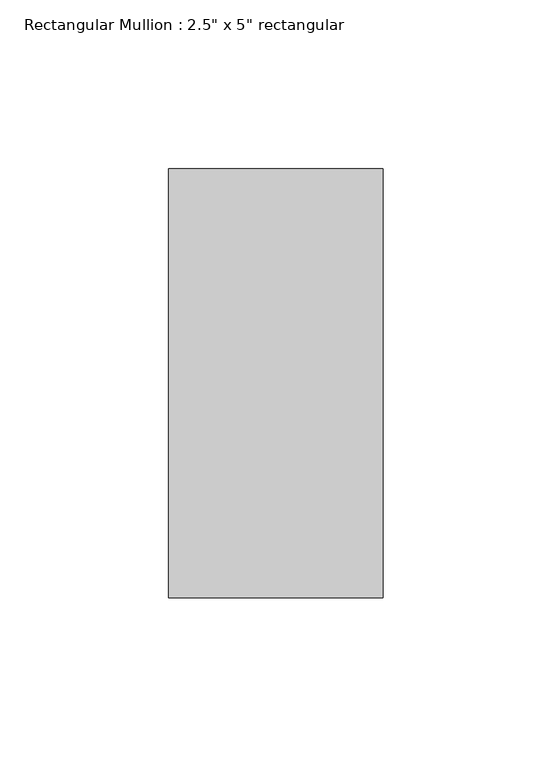
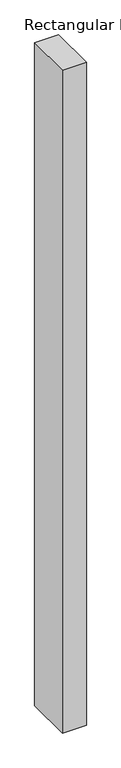
"""IFC4 building model written with IfcOpenShell, lengths in millimetres: member geometry."""

from ifc_helpers import new_model, si_unit, frame, origin, place, context, project, spatial, polyline, outline, extrude, source, transform, mapped, element, save


def member_b3eff8b9(model_context):
    return source(origin(), model_context, "Body", "SweptSolid", [
        extrude(outline(polyline([(0.0, 63.5), (0.0, -63.5), (-63.5, -63.5), (-63.5, 63.5), (0.0, 63.5)])), frame((0.0, 0.0, -1855.6083676), z_axis=(0.0, 0.0, 1.0), x_axis=(1.0, 0.0, 0.0)), (0.0, 0.0, 1.0), 1855.6083676),
    ])


if __name__ == "__main__":
    model = new_model("IFC4")
    model_context = context("Model", 3, world=origin())
    ifc_project = project(units=[si_unit("LENGTHUNIT", "METRE", prefix="MILLI")], contexts=[model_context])
    site = spatial("IfcSite", under=ifc_project)
    building = spatial("IfcBuilding", under=site)
    placement = place(None, origin())
    member_shape = member_b3eff8b9(model_context)
    element("IfcMember", 1, ObjectType="Rectangular Mullion : 2.5\" x 5\" rectangular", at=placement, inside=building, context=model_context, shape_type="MappedRepresentation", body=[
        mapped(member_shape, transform((0.0, 0.0, 0.0), x_axis=(1.0, 0.0, 0.0), y_axis=(0.0, 1.0, 0.0), z_axis=(0.0, 0.0, 1.0))),
    ])
    save(model, "model.ifc")

# Revit data of these elements
# Type "Rectangular Mullion : 2.5\" x 5\" rectangular"
#   built-in parameter 1007304 = 0.416667 (stored number, unit not read)
#   built-in parameter 1007301 = 0.104167 (stored number, unit not read)
#   built-in parameter 1007300 = 0.104167 (stored number, unit not read)
# Element 1 (IfcMember, "Rectangular Mullion : 2.5\" x 5\" rectangular")
#   Materials on its faces: "Aluminum"
# Materials
#   "Aluminum": class "Metal", colour RGB 247 247 247, transparency 0, Description = "Aluminum 6061", Cost = 0
